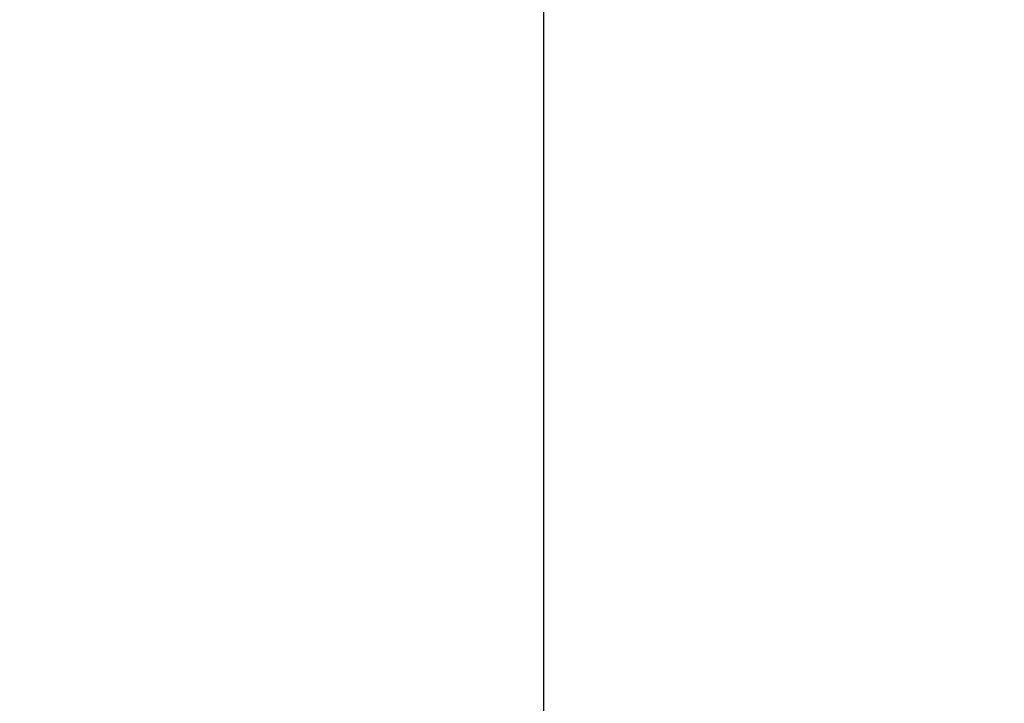
# Model space of a CAD drawing. Units: inches. Extents: x -48 to 50072, y 0 to 21068.
# Tile 15 of 75: x 163 to 263, y 347 to 417. Entities that reach past the tile are written whole.
import ezdxf

# ---------------------------------------------------------------- set-up
doc = ezdxf.new("R2010")
doc.units = ezdxf.units.IN
doc.header["$MEASUREMENT"] = 0
doc.layers.add('A-ANNO-DIMS', color=2, linetype='Continuous', lineweight=18)
doc.styles.get("Standard").update_dxf_attribs({"font": 'arial.ttf'})
doc.dimstyles.get("Standard").update_dxf_attribs({"dimtxt": 8, "dimasz": 0.18, "dimexe": 0.18, "dimexo": 0.0625, "dimgap": 0.09, "dimtad": 0, "dimtih": 1, "dimtoh": 1, "dimdec": 1, "dimzin": 0, "dimdsep": 46, "dimlunit": 4, "dimtxsty": 'Standard', "dimblk": 'ARCHTICK', "dimcen": 0.09, "dimadec": 0, "dimazin": 0, "dimtfac": 1, "dimtdec": 1, "dimtofl": 0, "dimtmove": 0, "dimatfit": 3, "dimldrblk": 'ARCHTICK', "dimfxl": 1, "dimtolj": 1, "dimtzin": 0, "dimarcsym": 0})

# ---------------------------------------------------------------- blocks, each defined once
blk = doc.blocks.new('_ArchTick')
at = {"color": 0, "linetype": 'ByBlock', "const_width": 0.15}
blk.add_lwpolyline([(-0.5, -0.5), (0.5, 0.5)], dxfattribs=at)
blk = doc.blocks.new('*D116')
at = {"layer": 'A-ANNO-DIMS', "color": 0, "lineweight": -2, "transparency": 16777216}
for p, q in [((18.017, 677.712), (18.017, 165.945)), ((216.017, 677.712), (216.017, 165.945)), ((18.017, 166.125), (108.458, 166.125)), ((216.017, 166.125), (125.576, 166.125))]:
    blk.add_line(p, q, dxfattribs=at)
at = {"layer": 'Defpoints', "color": 0, "transparency": 16777216}
for p in [(18.017, 677.775), (216.017, 677.775), (216.017, 166.125)]:
    blk.add_point(p, dxfattribs=at)
at = {"layer": 'A-ANNO-DIMS', "color": 0, "lineweight": -2, "transparency": 16777216, "xscale": 0.18, "yscale": 0.18, "zscale": 0.18, "rotation": 180}
blk.add_blockref('_ArchTick', (18.017, 166.125), dxfattribs=at)
at = {"layer": 'A-ANNO-DIMS', "color": 0, "lineweight": -2, "transparency": 16777216, "xscale": 0.18, "yscale": 0.18, "zscale": 0.18}
blk.add_blockref('_ArchTick', (216.017, 166.125), dxfattribs=at)
at = {"layer": 'A-ANNO-DIMS', "color": 0, "transparency": 16777216, "insert": (117.017, 166.125), "char_height": 8, "attachment_point": 5}
blk.add_mtext('\\A1;198', dxfattribs=at)
blk = doc.blocks.new('*D117')
at = {"layer": 'A-ANNO-DIMS', "color": 0, "lineweight": -2, "transparency": 16777216}
for p, q in [((216.017, 488.712), (216.017, 165.945)), ((297.017, 488.712), (297.017, 165.945)), ((216.017, 166.125), (251.464, 166.125)), ((297.017, 166.125), (261.57, 166.125))]:
    blk.add_line(p, q, dxfattribs=at)
at = {"layer": 'Defpoints', "color": 0, "transparency": 16777216}
for p in [(216.017, 488.775), (297.017, 488.775), (297.017, 166.125)]:
    blk.add_point(p, dxfattribs=at)
at = {"layer": 'A-ANNO-DIMS', "color": 0, "lineweight": -2, "transparency": 16777216, "xscale": 0.18, "yscale": 0.18, "zscale": 0.18, "rotation": 180}
blk.add_blockref('_ArchTick', (216.017, 166.125), dxfattribs=at)
at = {"layer": 'A-ANNO-DIMS', "color": 0, "lineweight": -2, "transparency": 16777216, "xscale": 0.18, "yscale": 0.18, "zscale": 0.18}
blk.add_blockref('_ArchTick', (297.017, 166.125), dxfattribs=at)
at = {"layer": 'A-ANNO-DIMS', "color": 0, "transparency": 16777216, "insert": (256.517, 166.125), "char_height": 8, "attachment_point": 5}
blk.add_mtext('\\A1;81', dxfattribs=at)

msp = doc.modelspace()

# ---------------------------------------------------------------- dimensions: what is measured, and where the dimension line sits
at = {"layer": 'A-ANNO-DIMS'}
for base, p1, p2, picture, middle in [((216.017, 166.125), (18.017, 677.775), (216.017, 677.775), '*D116', (117.017, 166.125)), ((297.017, 166.125), (216.017, 488.775), (297.017, 488.775), '*D117', (256.517, 166.125))]:
    dim = msp.add_linear_dim(base=base, p1=p1, p2=p2, dimstyle='Standard', override={"dimdec": 0, "dimlfac": 1, "dimrnd": 0, "dimzin": 0, "dimdsep": 46, "dimlunit": 2}, dxfattribs=at)
    dim.commit()
    dim.dimension.update_dxf_attribs({"geometry": picture, "text_midpoint": middle})

doc.saveas('drawing.dxf')
